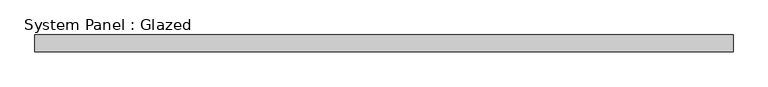
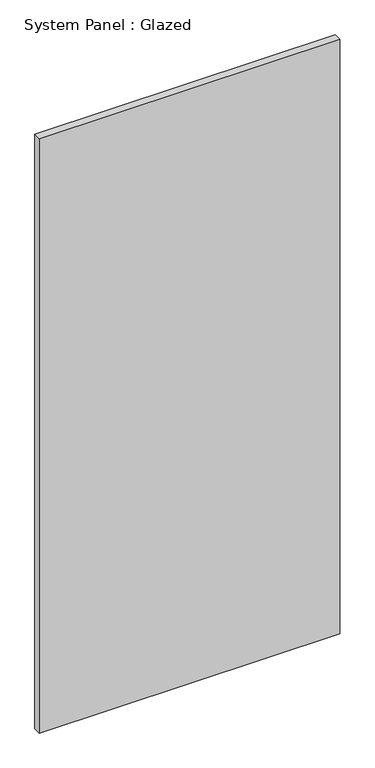
"""IFC4 building model written with IfcOpenShell, lengths in millimetres: plate geometry, System Panel : Glazed."""

from ifc_helpers import new_model, si_unit, origin, origin_with_axes, place, context, project, spatial, polyline, outline, extrude, source, transform, mapped, element, save


def system_panel_glazed_eda788cd(model_context):
    return source(origin(), model_context, "Body", "SweptSolid", [
        extrude(outline(polyline([(523.875, 19.05), (-523.875, 19.05), (-523.875, 44.45), (523.875, 44.45), (523.875, 19.05)])), origin_with_axes(), (0.0, 0.0, 1.0), 2190.75),
    ])


if __name__ == "__main__":
    model = new_model("IFC4")
    model_context = context("Model", 3, world=origin())
    ifc_project = project(units=[si_unit("LENGTHUNIT", "METRE", prefix="MILLI")], contexts=[model_context])
    site = spatial("IfcSite", under=ifc_project)
    building = spatial("IfcBuilding", under=site)
    placement = place(None, origin())
    system_panel_glazed_shape = system_panel_glazed_eda788cd(model_context)
    element("IfcPlate", 1, ObjectType="System Panel : Glazed", at=placement, inside=building, context=model_context, shape_type="MappedRepresentation", body=[
        mapped(system_panel_glazed_shape, transform((0.0, 0.0, 0.0), x_axis=(1.0, 0.0, 0.0), y_axis=(0.0, 1.0, 0.0), z_axis=(0.0, 0.0, 1.0))),
    ])
    save(model, "model.ifc")

# Revit data of these elements
# Type "System Panel : Glazed"
#   Construction Type Id = "GSP4R"
#   Analytic Construction = "1/8 in Pilkington single glazing"
#   Visual Light Transmittance = 0.9
#   Solar Heat Gain Coefficient = 0.86
#   Heat Transfer Coefficient (U) = 1.18115 BTU/(h·ft²·°F)
#   Define Thermal Properties by = 1
# Element 1 (IfcPlate, "System Panel : Glazed")
#   Materials on its faces: "Glass"
# Materials
#   "Glass": class "Glass", colour RGB 0 128 192, transparency 0.75, Description = "Soda Lime Glass", Cost = 0
